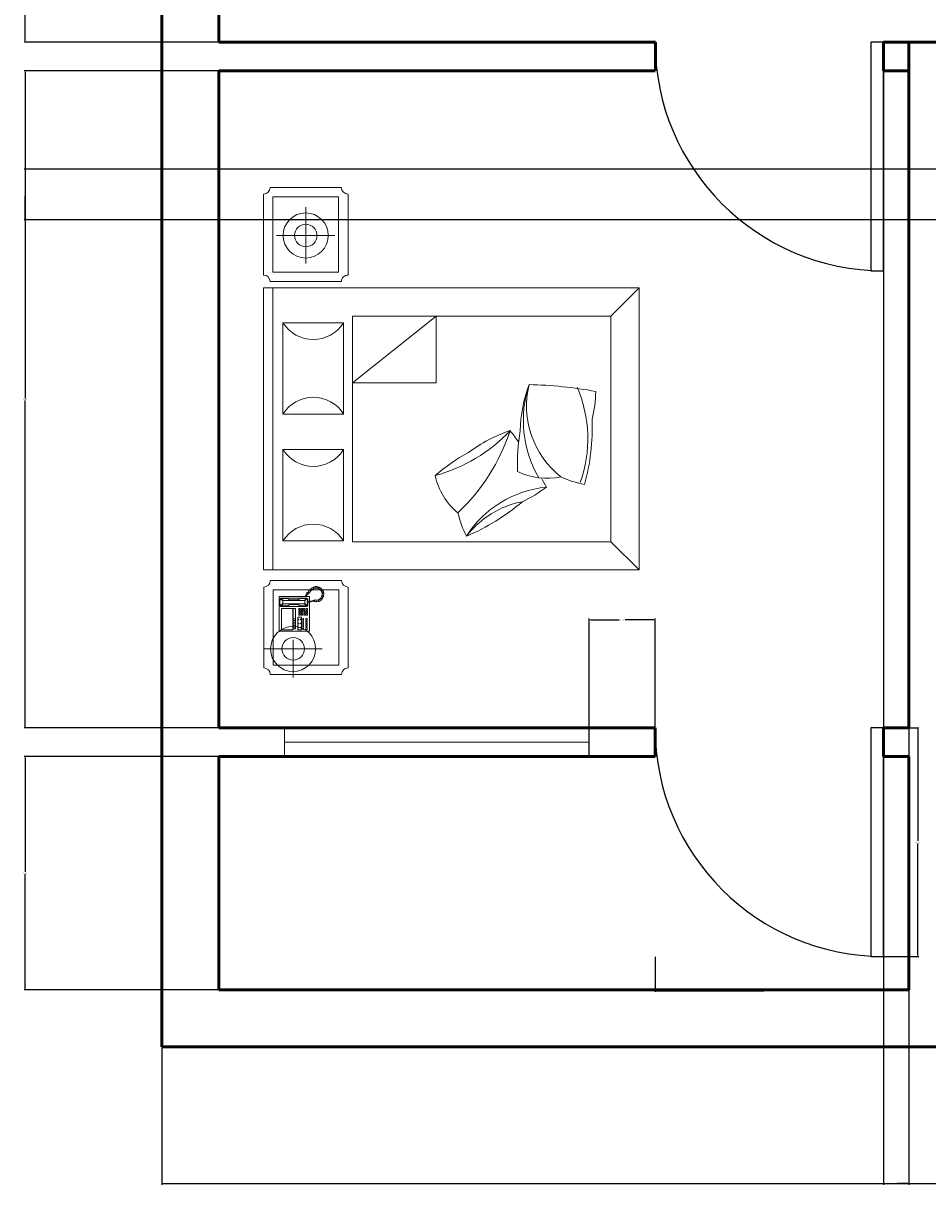
# Model space of a CAD drawing. Units: inches. Extents: x -108 to 1456, y -102 to 617.
# Tile 2 of 8: x 205 to 347, y 154 to 337. Entities that reach past the tile are written whole.
import ezdxf

# ---------------------------------------------------------------- set-up
doc = ezdxf.new("R2010")
doc.units = ezdxf.units.IN
for name, color, linetype, lineweight in [('A-ANNO-DIMS', 2, 'Continuous', 18), ('A-DOOR', 3, 'Continuous', 25), ('A-FURN', 8, 'Continuous', 18), ('A-GLAZ', 4, 'Continuous', 18), ('A-WALL', 7, 'Continuous', 50)]:
    doc.layers.add(name, color=color, linetype=linetype, lineweight=lineweight)
doc.styles.get("Standard").update_dxf_attribs({"font": 'arial.ttf'})
doc.dimstyles.get("Standard").update_dxf_attribs({"dimtxt": 0.18, "dimasz": 0.18, "dimexe": 0.18, "dimexo": 0.0625, "dimgap": 0.09, "dimtad": 0, "dimtih": 1, "dimtoh": 1, "dimdec": 4, "dimzin": 0, "dimdsep": 46, "dimtxsty": 'Standard', "dimcen": 0.09, "dimadec": 0, "dimazin": 0, "dimtfac": 1, "dimtdec": 4, "dimtofl": 0, "dimtmove": 0, "dimatfit": 3, "dimfxl": 1, "dimtolj": 1, "dimtzin": 0, "dimarcsym": 0})

# ---------------------------------------------------------------- blocks, each defined once
blk = doc.blocks.new('A$C50B66110')
for p, q in [((0.0503, 1.9981), (0.4803, 1.9981)), ((0.1513, 1.6871), (0.1513, 1.9967)), ((0.5716, 1.9488), (0.5716, 2)), ((0.5716, 2), (2.0719, 2)), ((2.0719, 1.9488), (2.0719, 2)), ((2.5701, 1.9993), (2.1401, 1.9993)), ((0.0153, 1.9631), (0.0153, 1.5831)), ((0.0653, 1.9481), (0.0653, 1.5981)), ((0.0653, 1.9481), (0.4653, 1.9481)), ((0.4653, 1.9481), (0.4653, 1.5981)), ((0.5153, 1.9631), (0.5153, 1.5831)), ((2.0719, 1.9488), (0.5716, 1.9488)), ((0.5716, 1.9488), (0.5716, 0)), ((2.0719, 0), (2.0719, 1.9488)), ((2.1051, 1.9643), (2.1051, 1.5843)), ((2.1551, 1.9493), (2.1551, 1.5993)), ((2.5551, 1.9493), (2.1551, 1.9493)), ((2.3505, 1.62), (2.3505, 1.9295)), ((2.5551, 1.9493), (2.5551, 1.5993)), ((2.6051, 1.9643), (2.6051, 1.5843)), ((0.7257, 1.5725), (0.7257, 1.8954)), ((0.7257, 1.8954), (1.2113, 1.8954)), ((1.2113, 1.8954), (1.2113, 1.5725)), ((1.4007, 1.5725), (1.4007, 1.8954)), ((1.4007, 1.8954), (1.8863, 1.8954)), ((1.8863, 1.8954), (1.8863, 1.5725)), ((0, 1.8416), (0.2001, 1.8416)), ((2.5018, 1.7744), (2.2017, 1.7744)), ((0.0503, 1.5481), (0.4803, 1.5481)), ((0.0653, 1.5981), (0.4653, 1.5981)), ((1.2113, 1.5725), (0.7257, 1.5725)), ((1.8863, 1.5725), (1.4007, 1.5725)), ((2.5701, 1.5493), (2.1401, 1.5493)), ((2.5551, 1.5993), (2.1551, 1.5993)), ((1.5665, 1.5254), (1.5665, 1.0802)), ((1.5665, 1.5254), (1.9219, 1.0802)), ((1.9219, 1.0802), (1.5665, 1.0802)), ((0.5716, 0), (0.7216, 0.15)), ((2.0719, 0), (1.9219, 0.15)), ((0.5716, 0), (2.0719, 0))]:
    blk.add_line(p, q)
at = {"linetype": 'ByBlock'}
for p, q in [((0.2481, 1.9162), (0.2458, 1.9139)), ((0.2481, 1.9162), (0.4287, 1.9162)), ((0.4287, 1.9162), (0.4309, 1.9139)), ((0.2458, 1.9139), (0.2458, 1.7562)), ((0.2526, 1.9036), (0.2526, 1.8431)), ((0.3669, 1.9036), (0.2526, 1.9036)), ((0.3669, 1.8431), (0.3669, 1.9036)), ((0.3772, 1.9071), (0.3818, 1.9128)), ((0.3772, 1.7688), (0.3772, 1.9071)), ((0.3818, 1.9094), (0.3807, 1.9048)), ((0.3807, 1.9048), (0.3807, 1.8739)), ((0.3807, 1.9048), (0.3909, 1.8945)), ((0.3807, 1.8739), (0.3829, 1.8682)), ((0.3818, 1.9128), (0.4161, 1.9128)), ((0.3864, 1.9116), (0.3818, 1.9094)), ((0.3829, 1.8682), (0.3864, 1.8625)), ((0.3921, 1.8968), (0.3864, 1.9116)), ((0.3864, 1.9116), (0.4138, 1.9116)), ((0.3864, 1.8625), (0.3875, 1.8545)), ((0.3875, 1.8545), (0.3875, 1.8431)), ((0.3909, 1.8945), (0.3921, 1.8968)), ((0.3909, 1.8431), (0.3909, 1.8945)), ((0.4081, 1.8968), (0.3921, 1.8968)), ((0.4081, 1.8968), (0.4138, 1.9116)), ((0.4092, 1.8945), (0.4081, 1.8968)), ((0.4195, 1.9048), (0.4092, 1.8945)), ((0.4092, 1.8431), (0.4092, 1.8945)), ((0.4138, 1.8625), (0.4127, 1.8545)), ((0.4127, 1.8545), (0.4127, 1.8431)), ((0.4138, 1.9116), (0.4184, 1.9094)), ((0.4172, 1.8682), (0.4138, 1.8625)), ((0.4161, 1.9128), (0.4218, 1.9071)), ((0.4195, 1.8739), (0.4172, 1.8682)), ((0.4184, 1.9094), (0.4195, 1.9048)), ((0.4195, 1.9048), (0.4195, 1.8739)), ((0.4218, 1.9071), (0.4218, 1.7699)), ((0.4309, 1.9139), (0.4309, 1.7562)), ((0.2526, 1.8431), (0.3669, 1.8431)), ((0.3201, 1.8168), (0.2526, 1.8168)), ((0.2526, 1.8168), (0.2526, 1.7962)), ((0.2526, 1.7962), (0.3201, 1.7962)), ((0.2572, 1.8408), (0.2572, 1.8294)), ((0.3669, 1.8408), (0.2572, 1.8408)), ((0.2572, 1.8294), (0.3669, 1.8294)), ((0.2675, 1.8145), (0.2641, 1.8145)), ((0.2641, 1.8145), (0.2641, 1.8111)), ((0.2641, 1.8111), (0.2675, 1.8111)), ((0.2641, 1.8019), (0.2641, 1.7985)), ((0.2675, 1.8019), (0.2641, 1.8019)), ((0.2641, 1.7985), (0.2675, 1.7985)), ((0.2664, 1.8408), (0.2664, 1.8294)), ((0.2675, 1.8111), (0.2675, 1.8145)), ((0.2675, 1.7985), (0.2675, 1.8019)), ((0.2755, 1.8408), (0.2755, 1.8294)), ((0.2846, 1.8408), (0.2846, 1.8294)), ((0.2846, 1.8145), (0.2846, 1.8111)), ((0.2881, 1.8145), (0.2846, 1.8145)), ((0.2846, 1.8111), (0.2881, 1.8111)), ((0.2846, 1.8019), (0.2846, 1.7985)), ((0.2881, 1.8019), (0.2846, 1.8019)), ((0.2846, 1.7985), (0.2881, 1.7985)), ((0.2881, 1.8111), (0.2881, 1.8145)), ((0.2881, 1.7985), (0.2881, 1.8019)), ((0.2938, 1.8408), (0.2938, 1.8294)), ((0.3029, 1.8408), (0.3029, 1.8294)), ((0.3052, 1.8145), (0.3052, 1.8111)), ((0.3086, 1.8145), (0.3052, 1.8145)), ((0.3052, 1.8111), (0.3086, 1.8111)), ((0.3052, 1.8019), (0.3052, 1.7985)), ((0.3086, 1.8019), (0.3052, 1.8019)), ((0.3052, 1.7985), (0.3086, 1.7985)), ((0.3086, 1.8111), (0.3086, 1.8145)), ((0.3086, 1.7985), (0.3086, 1.8019)), ((0.3121, 1.8408), (0.3121, 1.8294)), ((0.3201, 1.7962), (0.3201, 1.8168)), ((0.3304, 1.8111), (0.3395, 1.8111)), ((0.3304, 1.8042), (0.3304, 1.8111)), ((0.3395, 1.8042), (0.3304, 1.8042)), ((0.3304, 1.7985), (0.3395, 1.7985)), ((0.3304, 1.7916), (0.3304, 1.7985)), ((0.3395, 1.8111), (0.3395, 1.8042)), ((0.3395, 1.7985), (0.3395, 1.7916)), ((0.3441, 1.8042), (0.3441, 1.8111)), ((0.3441, 1.8111), (0.3532, 1.8111)), ((0.3532, 1.8042), (0.3441, 1.8042)), ((0.3441, 1.7985), (0.3532, 1.7985)), ((0.3441, 1.7916), (0.3441, 1.7985)), ((0.3532, 1.8111), (0.3532, 1.8042)), ((0.3532, 1.7985), (0.3532, 1.7916)), ((0.3578, 1.8111), (0.3669, 1.8111)), ((0.3578, 1.8042), (0.3578, 1.8111)), ((0.3669, 1.8042), (0.3578, 1.8042)), ((0.3578, 1.7985), (0.3669, 1.7985)), ((0.3578, 1.7916), (0.3578, 1.7985)), ((0.3669, 1.8294), (0.3669, 1.8408)), ((0.3669, 1.8111), (0.3669, 1.8042)), ((0.3669, 1.7985), (0.3669, 1.7916)), ((0.3807, 1.8019), (0.3829, 1.8076)), ((0.3807, 1.7711), (0.3807, 1.8019)), ((0.3829, 1.8076), (0.3864, 1.8134)), ((0.3864, 1.8134), (0.3875, 1.8214)), ((0.3875, 1.8214), (0.3875, 1.8431)), ((0.3909, 1.8431), (0.3909, 1.7813)), ((0.4092, 1.8431), (0.4092, 1.7813)), ((0.4127, 1.8214), (0.4127, 1.8431)), ((0.4138, 1.8134), (0.4127, 1.8214)), ((0.4172, 1.8076), (0.4138, 1.8134)), ((0.4195, 1.8019), (0.4172, 1.8076)), ((0.4195, 1.7711), (0.4195, 1.8019)), ((0.2458, 1.7562), (0.2481, 1.7539)), ((0.4, 1.7539), (0.2481, 1.7539)), ((0.2652, 1.7905), (0.2538, 1.7905)), ((0.2538, 1.7905), (0.2538, 1.7859)), ((0.2538, 1.7859), (0.2652, 1.7859)), ((0.2538, 1.7665), (0.2538, 1.7733)), ((0.2538, 1.7733), (0.2652, 1.7733)), ((0.2652, 1.7665), (0.2538, 1.7665)), ((0.2652, 1.7859), (0.2652, 1.7905)), ((0.2652, 1.7733), (0.2652, 1.7665)), ((0.2812, 1.7905), (0.2698, 1.7905)), ((0.2698, 1.7905), (0.2698, 1.7859)), ((0.2698, 1.7859), (0.2812, 1.7859)), ((0.2698, 1.7665), (0.2698, 1.7733)), ((0.2698, 1.7733), (0.2812, 1.7733)), ((0.2812, 1.7665), (0.2698, 1.7665)), ((0.2812, 1.7859), (0.2812, 1.7905)), ((0.2812, 1.7733), (0.2812, 1.7665)), ((0.2972, 1.7905), (0.2858, 1.7905)), ((0.2858, 1.7905), (0.2858, 1.7859)), ((0.2858, 1.7859), (0.2972, 1.7859)), ((0.2858, 1.7665), (0.2858, 1.7733)), ((0.2858, 1.7733), (0.2972, 1.7733)), ((0.2972, 1.7665), (0.2858, 1.7665)), ((0.2972, 1.7859), (0.2972, 1.7905)), ((0.2972, 1.7733), (0.2972, 1.7665)), ((0.3018, 1.7905), (0.3018, 1.7859)), ((0.3132, 1.7905), (0.3018, 1.7905)), ((0.3018, 1.7859), (0.3132, 1.7859)), ((0.3018, 1.7733), (0.3132, 1.7733)), ((0.3018, 1.7665), (0.3018, 1.7733)), ((0.3132, 1.7665), (0.3018, 1.7665)), ((0.3132, 1.7859), (0.3132, 1.7905)), ((0.3132, 1.7733), (0.3132, 1.7665)), ((0.3395, 1.7916), (0.3304, 1.7916)), ((0.3304, 1.7779), (0.3304, 1.7848)), ((0.3304, 1.7848), (0.3395, 1.7848)), ((0.3395, 1.7779), (0.3304, 1.7779)), ((0.3304, 1.7722), (0.3395, 1.7722)), ((0.3304, 1.7653), (0.3304, 1.7722)), ((0.3395, 1.7653), (0.3304, 1.7653)), ((0.3395, 1.7848), (0.3395, 1.7779)), ((0.3395, 1.7722), (0.3395, 1.7653)), ((0.3532, 1.7916), (0.3441, 1.7916)), ((0.3441, 1.7779), (0.3441, 1.7848)), ((0.3441, 1.7848), (0.3532, 1.7848)), ((0.3532, 1.7779), (0.3441, 1.7779)), ((0.3441, 1.7722), (0.3532, 1.7722)), ((0.3441, 1.7653), (0.3441, 1.7722)), ((0.3532, 1.7653), (0.3441, 1.7653)), ((0.3532, 1.7848), (0.3532, 1.7779)), ((0.3532, 1.7722), (0.3532, 1.7653)), ((0.3669, 1.7916), (0.3578, 1.7916)), ((0.3578, 1.7791), (0.3578, 1.7859)), ((0.3578, 1.7859), (0.3669, 1.7859)), ((0.3669, 1.7791), (0.3578, 1.7791)), ((0.3578, 1.7653), (0.3578, 1.7722)), ((0.3578, 1.7722), (0.3669, 1.7722)), ((0.3669, 1.7653), (0.3578, 1.7653)), ((0.3669, 1.7859), (0.3669, 1.7791)), ((0.3669, 1.7722), (0.3669, 1.7653)), ((0.3829, 1.7631), (0.3772, 1.7688)), ((0.3807, 1.7711), (0.3909, 1.7813)), ((0.3818, 1.7665), (0.3807, 1.7711)), ((0.3864, 1.7642), (0.3818, 1.7665)), ((0.399, 1.7631), (0.3829, 1.7631)), ((0.3921, 1.7791), (0.3864, 1.7642)), ((0.3864, 1.7642), (0.399, 1.7642)), ((0.3909, 1.7813), (0.3921, 1.7791)), ((0.4081, 1.7791), (0.3921, 1.7791)), ((0.4024, 1.7676), (0.3989, 1.7676)), ((0.3989, 1.7676), (0.3991, 1.7578)), ((0.3991, 1.7578), (0.4019, 1.7462)), ((0.4019, 1.7462), (0.4047, 1.7353)), ((0.403, 1.7585), (0.4024, 1.7676)), ((0.4026, 1.7642), (0.4138, 1.7642)), ((0.4161, 1.7631), (0.4027, 1.7631)), ((0.4047, 1.7511), (0.403, 1.7585)), ((0.4287, 1.7539), (0.404, 1.7539)), ((0.4047, 1.7353), (0.4044, 1.7293)), ((0.4074, 1.7402), (0.4047, 1.7511)), ((0.4081, 1.7346), (0.4074, 1.7402)), ((0.4079, 1.7286), (0.4081, 1.7346)), ((0.4092, 1.7813), (0.4081, 1.7791)), ((0.4081, 1.7791), (0.4138, 1.7642)), ((0.4195, 1.7711), (0.4092, 1.7813)), ((0.4138, 1.7642), (0.4184, 1.7665)), ((0.4218, 1.7699), (0.4161, 1.7631)), ((0.4184, 1.7665), (0.4195, 1.7711)), ((0.4309, 1.7562), (0.4287, 1.7539)), ((0.4378, 1.7742), (0.4309, 1.7768)), ((0.4309, 1.7722), (0.436, 1.7708)), ((0.436, 1.7708), (0.4406, 1.7672)), ((0.441, 1.771), (0.4378, 1.7742)), ((0.4406, 1.7672), (0.4418, 1.7656)), ((0.4434, 1.7688), (0.441, 1.771)), ((0.4443, 1.7658), (0.4418, 1.7633)), ((0.4418, 1.7656), (0.4443, 1.7658)), ((0.4418, 1.7633), (0.4511, 1.7551)), ((0.4477, 1.7704), (0.4434, 1.7688)), ((0.4497, 1.7684), (0.4477, 1.7704)), ((0.4481, 1.765), (0.4497, 1.7684)), ((0.4509, 1.7672), (0.4481, 1.765)), ((0.4539, 1.764), (0.4509, 1.7672)), ((0.4511, 1.7551), (0.4662, 1.7422)), ((0.4515, 1.7573), (0.4539, 1.764)), ((0.4577, 1.7605), (0.4515, 1.7573)), ((0.463, 1.7555), (0.4577, 1.7605)), ((0.4618, 1.7482), (0.463, 1.7555)), ((0.467, 1.7515), (0.4618, 1.7482)), ((0.4664, 1.7418), (0.4741, 1.72)), ((0.4714, 1.7468), (0.467, 1.7515)), ((0.4696, 1.7418), (0.4714, 1.7468)), ((0.4766, 1.7425), (0.4697, 1.7418)), ((0.472, 1.733), (0.4787, 1.7356)), ((0.4794, 1.7332), (0.472, 1.733)), ((0.4787, 1.7356), (0.4766, 1.7425)), ((0.481, 1.7279), (0.4794, 1.7332)), ((0.4026, 1.7254), (0.4021, 1.7198)), ((0.4021, 1.7198), (0.4088, 1.7187)), ((0.4088, 1.7187), (0.4023, 1.7147)), ((0.4023, 1.7147), (0.4028, 1.7085)), ((0.4051, 1.7279), (0.4026, 1.7254)), ((0.4028, 1.7085), (0.4102, 1.7078)), ((0.4102, 1.7078), (0.4037, 1.7027)), ((0.4037, 1.7027), (0.4067, 1.6974)), ((0.4044, 1.7293), (0.4051, 1.7279)), ((0.4067, 1.6974), (0.4137, 1.6988)), ((0.4121, 1.7256), (0.4079, 1.7286)), ((0.4137, 1.6988), (0.4104, 1.6923)), ((0.4104, 1.6923), (0.4139, 1.6881)), ((0.4111, 1.7203), (0.4121, 1.7256)), ((0.4123, 1.7057), (0.4111, 1.7203)), ((0.4211, 1.6946), (0.4123, 1.7057)), ((0.4139, 1.6881), (0.4192, 1.692)), ((0.4192, 1.692), (0.4183, 1.6858)), ((0.4183, 1.6858), (0.4227, 1.683)), ((0.4333, 1.6881), (0.4211, 1.6946)), ((0.4227, 1.683), (0.4283, 1.6876)), ((0.4283, 1.6876), (0.4276, 1.68)), ((0.4276, 1.68), (0.4324, 1.6786)), ((0.4324, 1.6786), (0.4354, 1.6849)), ((0.4472, 1.6869), (0.4333, 1.6881)), ((0.4354, 1.6849), (0.4382, 1.6786)), ((0.4382, 1.6786), (0.4421, 1.6782)), ((0.4421, 1.6782), (0.4437, 1.6849)), ((0.4437, 1.6849), (0.4463, 1.6775)), ((0.4463, 1.6775), (0.4507, 1.6786)), ((0.4606, 1.6927), (0.4472, 1.6869)), ((0.4507, 1.6786), (0.4509, 1.6849)), ((0.4509, 1.6849), (0.4562, 1.6802)), ((0.4562, 1.6802), (0.4599, 1.6821)), ((0.4592, 1.689), (0.4641, 1.683)), ((0.4599, 1.6821), (0.4592, 1.689)), ((0.4708, 1.7027), (0.4606, 1.6927)), ((0.4641, 1.683), (0.4678, 1.6863)), ((0.465, 1.6925), (0.4715, 1.6897)), ((0.4678, 1.6863), (0.465, 1.6925)), ((0.4741, 1.72), (0.4708, 1.7027)), ((0.4745, 1.6925), (0.4713, 1.6988)), ((0.4713, 1.6988), (0.478, 1.6967)), ((0.4715, 1.6897), (0.4745, 1.6925)), ((0.4743, 1.7075), (0.4815, 1.7073)), ((0.4798, 1.7013), (0.4743, 1.7075)), ((0.4761, 1.7233), (0.481, 1.7279)), ((0.4824, 1.7233), (0.4761, 1.7233)), ((0.4764, 1.7154), (0.4835, 1.7175)), ((0.4824, 1.7119), (0.4764, 1.7154)), ((0.478, 1.6967), (0.4798, 1.7013)), ((0.4815, 1.7073), (0.4824, 1.7119)), ((0.4835, 1.7175), (0.4824, 1.7233)), ((0.7216, 1.5254), (1.9219, 1.5254)), ((0.7216, 1.5254), (0.7216, 0.15)), ((1.9219, 0.15), (1.9219, 1.5254)), ((0.7216, 0.15), (1.9219, 0.15))]:
    blk.add_line(p, q, dxfattribs=at)
for centre, radius in [((0.1513, 1.8416), 0.12), ((0.1513, 1.8416), 0.06), ((2.3505, 1.7744), 0.12), ((2.3505, 1.7744), 0.06)]:
    blk.add_circle(centre, radius)
for centre, radius, start, end in [((0.0153, 1.9981), 0.035, 270, 0), ((0.5153, 1.9981), 0.035, 180, 270), ((2.1051, 1.9993), 0.035, 270, 0), ((2.6051, 1.9993), 0.035, 180, 270), ((0.6244, 1.734), 0.1906, 302.12017, 57.87983), ((1.3126, 1.734), 0.1906, 122.12017, 237.87983), ((1.2994, 1.734), 0.1906, 302.12017, 57.87983), ((1.9876, 1.734), 0.1906, 122.12017, 237.87983), ((0.0153, 1.5481), 0.035, 0, 90), ((0.5153, 1.5481), 0.035, 90, 180), ((2.1051, 1.5493), 0.035, 0, 90), ((2.6051, 1.5493), 0.035, 90, 180), ((1.1502, 0.7366), 0.3575, 102.47819, 140.46254), ((0.328, 0.4368), 0.9879, 28.49711, 41.05657), ((1.9117, 1.3157), 0.8697, 195.33601, 226.41927), ((0.9996, 0.4307), 0.548, 103.20343, 117.03623), ((1.656, 1.7093), 1.0798, 223.63057, 251.4288), ((0.4482, 0.4408), 0.5655, 5.33912, 57.68949), ((1.8226, 1.3753), 1.1652, 203.06416, 220.32086), ((0.4548, 0.5307), 0.4879, 10.69865, 52.68638), ((0.5648, 0.4378), 0.7874, 18.35266, 36.68512), ((-0.0179, 2.4352), 2.1977, 305.29657, 307.24182), ((1.5981, 0.9345), 0.734, 205.25901, 216.93514), ((1.4166, 0.4903), 0.3575, 154.0418, 192.02615), ((1.1403, -0.3401), 0.9879, 80.06073, 92.62018), ((1.2867, -0.154), 0.7874, 69.91627, 88.24873), ((1.3672, 0.0075), 0.6085, 71.81005, 120.13512), ((1.4431, 0.1219), 0.4774, 76.18494, 142.00166), ((-0.6401, 0.6314), 2.1977, 349.48843, 358.80544), ((-0.0179, 2.4352), 2.1977, 297.92482, 299.3793), ((1.5626, 0.1822), 0.548, 154.76704, 168.59984), ((1.2678, 0.9611), 0.6885, 250.29361, 293.6414), ((1.3343, 1.4141), 1.1652, 254.62778, 271.88448), ((1.5399, 0.9642), 0.734, 256.82263, 268.49876)]:
    blk.add_arc(centre, radius, start, end)
blk = doc.blocks.new('DOOR-36-SWING')
for p, q in [((36, 36), (34, 36)), ((34, 36), (34, 0)), ((36, 36), (34, 36)), ((36, 0), (36, 36)), ((34, 0), (36, 0))]:
    blk.add_line(p, q)
blk.add_arc((36, 36), 36, 180, 270)
blk = doc.blocks.new('WIN-48-WALL-4_5')
for p, q in [((0, 0), (0, 4.5)), ((48, 0), (48, 4.5)), ((0, 2.25), (48, 2.25))]:
    blk.add_line(p, q)
blk = doc.blocks.new('*D12')
at = {"layer": 'A-ANNO-DIMS', "color": 0, "lineweight": -2, "transparency": 16777216}
for p, q in [((304.09, 189.96), (304.09, 184.44)), ((340.09, 189.96), (340.09, 184.44)), ((304.27, 184.62), (321.16, 184.62)), ((339.91, 184.62), (323.03, 184.62))]:
    blk.add_line(p, q, dxfattribs=at)
at = {"layer": 'A-ANNO-DIMS', "color": 0, "transparency": 16777216}
for points in [[(304.27, 184.65), (304.27, 184.59), (304.09, 184.62)], [(339.91, 184.65), (339.91, 184.59), (340.09, 184.62)]]:
    blk.add_solid(points, dxfattribs=at)
at = {"layer": 'Defpoints', "color": 0, "transparency": 16777216}
for p in [(304.09, 190.02), (340.09, 190.02), (340.09, 184.62)]:
    blk.add_point(p, dxfattribs=at)
at = {"layer": 'A-ANNO-DIMS', "color": 0, "transparency": 16777216, "insert": (322.09, 184.62), "char_height": 0.18, "attachment_point": 5}
blk.add_mtext('\\A1;DOOR 36 TYP.', dxfattribs=at)
blk = doc.blocks.new('*D13')
at = {"layer": 'A-ANNO-DIMS', "color": 0, "lineweight": -2, "transparency": 16777216}
for p, q in [((340.16, 226.02), (345.67, 226.02)), ((345.49, 225.84), (345.49, 208.21)), ((345.49, 190.2), (345.49, 207.84)), ((340.16, 190.02), (345.67, 190.02))]:
    blk.add_line(p, q, dxfattribs=at)
at = {"layer": 'A-ANNO-DIMS', "color": 0, "transparency": 16777216}
for points in [[(345.46, 225.84), (345.52, 225.84), (345.49, 226.02)], [(345.46, 190.2), (345.52, 190.2), (345.49, 190.02)]]:
    blk.add_solid(points, dxfattribs=at)
at = {"layer": 'Defpoints', "color": 0, "transparency": 16777216}
for p in [(340.09, 226.02), (345.49, 226.02), (340.09, 190.02)]:
    blk.add_point(p, dxfattribs=at)
at = {"layer": 'A-ANNO-DIMS', "color": 0, "transparency": 16777216, "insert": (345.49, 208.02), "char_height": 0.18, "attachment_point": 5}
blk.add_mtext('\\A1;36 TYP.', dxfattribs=at)
blk = doc.blocks.new('*D34')
at = {"layer": 'A-ANNO-DIMS', "color": 0, "lineweight": -2, "transparency": 16777216}
for p, q in [((226.34, 175.71), (226.34, 154.07)), ((538.34, 175.71), (538.34, 154.07)), ((226.52, 154.25), (382.06, 154.25)), ((538.16, 154.25), (382.63, 154.25))]:
    blk.add_line(p, q, dxfattribs=at)
at = {"layer": 'A-ANNO-DIMS', "color": 0, "transparency": 16777216}
for points in [[(226.52, 154.28), (226.52, 154.22), (226.34, 154.25)], [(538.16, 154.28), (538.16, 154.22), (538.34, 154.25)]]:
    blk.add_solid(points, dxfattribs=at)
at = {"layer": 'Defpoints', "color": 0, "transparency": 16777216}
for p in [(226.34, 175.77), (538.34, 175.77), (538.34, 154.25)]:
    blk.add_point(p, dxfattribs=at)
at = {"layer": 'A-ANNO-DIMS', "color": 0, "transparency": 16777216, "insert": (382.34, 154.25), "char_height": 0.18, "attachment_point": 5}
blk.add_mtext('\\A1;312', dxfattribs=at)
blk = doc.blocks.new('*D40')
at = {"layer": 'A-ANNO-DIMS', "color": 0, "lineweight": -2, "transparency": 16777216}
for p, q in [((235.28, 449.52), (204.64, 449.52)), ((204.82, 449.34), (204.82, 391.96)), ((204.82, 334.2), (204.82, 391.59)), ((235.28, 334.02), (204.64, 334.02))]:
    blk.add_line(p, q, dxfattribs=at)
at = {"layer": 'A-ANNO-DIMS', "color": 0, "transparency": 16777216}
for points in [[(204.79, 449.34), (204.85, 449.34), (204.82, 449.52)], [(204.79, 334.2), (204.85, 334.2), (204.82, 334.02)]]:
    blk.add_solid(points, dxfattribs=at)
at = {"layer": 'Defpoints', "color": 0, "transparency": 16777216}
for p in [(235.34, 449.52), (204.82, 334.02), (235.34, 334.02)]:
    blk.add_point(p, dxfattribs=at)
at = {"layer": 'A-ANNO-DIMS', "color": 0, "transparency": 16777216, "insert": (204.82, 391.77), "char_height": 0.18, "attachment_point": 5}
blk.add_mtext('\\A1;115.5', dxfattribs=at)
blk = doc.blocks.new('*D41')
at = {"layer": 'A-ANNO-DIMS', "color": 0, "lineweight": -2, "transparency": 16777216}
for p, q in [((235.28, 329.52), (204.64, 329.52)), ((204.82, 329.34), (204.82, 277.96)), ((204.82, 226.2), (204.82, 277.59)), ((235.28, 226.02), (204.64, 226.02))]:
    blk.add_line(p, q, dxfattribs=at)
at = {"layer": 'A-ANNO-DIMS', "color": 0, "transparency": 16777216}
for points in [[(204.79, 329.34), (204.85, 329.34), (204.82, 329.52)], [(204.79, 226.2), (204.85, 226.2), (204.82, 226.02)]]:
    blk.add_solid(points, dxfattribs=at)
at = {"layer": 'Defpoints', "color": 0, "transparency": 16777216}
for p in [(235.34, 329.52), (204.82, 226.02), (235.34, 226.02)]:
    blk.add_point(p, dxfattribs=at)
at = {"layer": 'A-ANNO-DIMS', "color": 0, "transparency": 16777216, "insert": (204.82, 277.77), "char_height": 0.18, "attachment_point": 5}
blk.add_mtext('\\A1;103.5', dxfattribs=at)
blk = doc.blocks.new('*D42')
at = {"layer": 'A-ANNO-DIMS', "color": 0, "lineweight": -2, "transparency": 16777216}
for p, q in [((235.28, 221.52), (204.64, 221.52)), ((204.82, 221.34), (204.82, 203.33)), ((204.82, 184.95), (204.82, 202.97)), ((235.28, 184.77), (204.64, 184.77))]:
    blk.add_line(p, q, dxfattribs=at)
at = {"layer": 'A-ANNO-DIMS', "color": 0, "transparency": 16777216}
for points in [[(204.79, 221.34), (204.85, 221.34), (204.82, 221.52)], [(204.79, 184.95), (204.85, 184.95), (204.82, 184.77)]]:
    blk.add_solid(points, dxfattribs=at)
at = {"layer": 'Defpoints', "color": 0, "transparency": 16777216}
for p in [(235.34, 221.52), (204.82, 184.77), (235.34, 184.77)]:
    blk.add_point(p, dxfattribs=at)
at = {"layer": 'A-ANNO-DIMS', "color": 0, "transparency": 16777216, "insert": (204.82, 203.15), "char_height": 0.18, "attachment_point": 5}
blk.add_mtext('\\A1;36.75', dxfattribs=at)
blk = doc.blocks.new('*D43')
at = {"layer": 'A-ANNO-DIMS', "color": 0, "lineweight": -2, "transparency": 16777216}
for p, q in [((340.09, 329.46), (340.09, 154.07)), ((344.09, 329.46), (344.09, 154.07)), ((340.27, 154.25), (341.94, 154.25)), ((343.91, 154.25), (342.25, 154.25))]:
    blk.add_line(p, q, dxfattribs=at)
at = {"layer": 'A-ANNO-DIMS', "color": 0, "transparency": 16777216}
for points in [[(340.27, 154.28), (340.27, 154.22), (340.09, 154.25)], [(343.91, 154.28), (343.91, 154.22), (344.09, 154.25)]]:
    blk.add_solid(points, dxfattribs=at)
at = {"layer": 'Defpoints', "color": 0, "transparency": 16777216}
for p in [(340.09, 329.52), (344.09, 329.52), (344.09, 154.25)]:
    blk.add_point(p, dxfattribs=at)
at = {"layer": 'A-ANNO-DIMS', "color": 0, "transparency": 16777216, "insert": (342.09, 154.25), "char_height": 0.18, "attachment_point": 5}
blk.add_mtext('\\A1;4', dxfattribs=at)
blk = doc.blocks.new('*D44')
at = {"layer": 'A-ANNO-DIMS', "color": 0, "lineweight": -2, "transparency": 16777216}
for p, q in [((293.72, 221.59), (293.72, 243.23)), ((293.9, 243.05), (298.45, 243.05)), ((303.91, 243.05), (299.36, 243.05)), ((304.09, 221.59), (304.09, 243.23))]:
    blk.add_line(p, q, dxfattribs=at)
at = {"layer": 'A-ANNO-DIMS', "color": 0, "transparency": 16777216}
for points in [[(293.9, 243.08), (293.9, 243.02), (293.72, 243.05)], [(303.91, 243.08), (303.91, 243.02), (304.09, 243.05)]]:
    blk.add_solid(points, dxfattribs=at)
at = {"layer": 'Defpoints', "color": 0, "transparency": 16777216}
for p in [(304.09, 243.05), (293.72, 221.52), (304.09, 221.52)]:
    blk.add_point(p, dxfattribs=at)
at = {"layer": 'A-ANNO-DIMS', "color": 0, "transparency": 16777216, "insert": (298.91, 243.05), "char_height": 0.18, "attachment_point": 5}
blk.add_mtext('\\A1;10.375', dxfattribs=at)
blk = doc.blocks.new('*D64')
at = {"layer": 'A-ANNO-DIMS', "color": 0, "lineweight": -2, "transparency": 16777216}
for p, q in [((348.53, 314.02), (204.64, 314.02)), ((204.82, 313.84), (204.82, 310.21)), ((204.82, 306.2), (204.82, 309.84)), ((348.53, 306.02), (204.64, 306.02))]:
    blk.add_line(p, q, dxfattribs=at)
at = {"layer": 'A-ANNO-DIMS', "color": 0, "transparency": 16777216}
for points in [[(204.79, 313.84), (204.85, 313.84), (204.82, 314.02)], [(204.79, 306.2), (204.85, 306.2), (204.82, 306.02)]]:
    blk.add_solid(points, dxfattribs=at)
at = {"layer": 'Defpoints', "color": 0, "transparency": 16777216}
for p in [(348.59, 314.02), (204.82, 306.02), (348.59, 306.02)]:
    blk.add_point(p, dxfattribs=at)
at = {"layer": 'A-ANNO-DIMS', "color": 0, "transparency": 16777216, "insert": (204.82, 310.02), "char_height": 0.18, "attachment_point": 5}
blk.add_mtext('\\A1;8', dxfattribs=at)

msp = doc.modelspace()

# ---------------------------------------------------------------- linework, layer by layer
at = {"layer": 'A-WALL'}
for p, q in [((226.3443, 595.7743), (226.3443, 175.7743)), ((235.3443, 334.0243), (235.3443, 449.5243)), ((235.3443, 449.5243), (235.3443, 334.0243)), ((304.0943, 334.0243), (235.3443, 334.0243)), ((304.1647, 334.0243), (304.0943, 334.0243)), ((304.1647, 329.5243), (304.1647, 334.0243)), ((344.0943, 334.0243), (340.0943, 334.0243)), ((340.0943, 329.5243), (340.0943, 334.0243)), ((344.0943, 334.0243), (344.0943, 226.0243)), ((344.0943, 329.5243), (344.0943, 334.0243)), ((344.0943, 334.0243), (348.5943, 334.0243)), ((304.0943, 329.5243), (235.3443, 329.5243)), ((235.3443, 329.5243), (235.3443, 226.0243)), ((344.0943, 329.5243), (340.0943, 329.5243)), ((304.0943, 226.0243), (235.3443, 226.0243)), ((304.0943, 221.5243), (304.0943, 226.0243)), ((344.0943, 226.0243), (340.0943, 226.0243)), ((340.0943, 221.5243), (340.0943, 226.0243)), ((304.0943, 221.5243), (235.3443, 221.5243)), ((235.3443, 221.5243), (304.0943, 221.5243)), ((235.3443, 221.5243), (235.3443, 184.7743)), ((344.0943, 221.5243), (340.0943, 221.5243)), ((344.0943, 221.5243), (344.0943, 184.7743)), ((235.3443, 184.7743), (344.0943, 184.7743)), ((226.3443, 175.7743), (538.3443, 175.7743))]:
    msp.add_line(p, q, dxfattribs=at)

# ---------------------------------------------------------------- block references
at = {"layer": 'A-DOOR'}
for p in [(304.094, 298.024), (304.094, 190.024)]:
    msp.add_blockref('DOOR-36-SWING', p, dxfattribs=at)
at = {"layer": 'A-FURN', "xscale": 29.60830491940187, "yscale": 29.60830491940187, "zscale": 29.60830491940187, "rotation": 89.99999999999991}
msp.add_blockref('A$C50B66110', (301.5751, 233.9822), dxfattribs=at)
at = {"layer": 'A-GLAZ'}
msp.add_blockref('WIN-48-WALL-4_5', (245.719, 221.524), dxfattribs=at)

# ---------------------------------------------------------------- dimensions: what is measured, and where the dimension line sits
at = {"layer": 'A-ANNO-DIMS'}
for base, p1, p2, override, picture, middle in [((204.8193, 334.0243), (235.3443, 449.5243), (235.3443, 334.0243), {"dimdec": 1, "dimlfac": 1, "dimrnd": 0, "dimzin": 0, "dimdsep": 46, "dimlunit": 2}, '*D40', (204.8193, 391.7743)), ((204.8193, 226.0243), (235.3443, 329.5243), (235.3443, 226.0243), {"dimdec": 1, "dimlfac": 1, "dimrnd": 0, "dimzin": 0, "dimdsep": 46, "dimlunit": 2}, '*D41', (204.8193, 277.7743)), ((204.8193, 306.0243), (348.5943, 314.0243), (348.5943, 306.0243), {"dimdec": 0, "dimlfac": 1, "dimrnd": 0, "dimzin": 0, "dimdsep": 46, "dimlunit": 2}, '*D64', (204.8193, 310.0243)), ((204.8193, 184.7743), (235.3443, 221.5243), (235.3443, 184.7743), {"dimdec": 2, "dimlfac": 1, "dimrnd": 0, "dimzin": 0, "dimdsep": 46, "dimlunit": 2}, '*D42', (204.8193, 203.1493))]:
    dim = msp.add_linear_dim(base=base, p1=p1, p2=p2, angle=90, dimstyle='Standard', override=override, dxfattribs=at)
    dim.commit()
    dim.dimension.update_dxf_attribs({"geometry": picture, "text_midpoint": middle})
for base, p1, p2, override, picture, middle in [((344.0943, 154.2493), (340.0943, 329.5243), (344.0943, 329.5243), {"dimdec": 0, "dimlfac": 1, "dimrnd": 0, "dimzin": 0, "dimdsep": 46, "dimlunit": 2}, '*D43', (342.0943, 154.2493)), ((304.0943, 243.0493), (293.7193, 221.5243), (304.0943, 221.5243), {"dimdec": 3, "dimlfac": 1, "dimrnd": 0, "dimzin": 0, "dimdsep": 46, "dimlunit": 2}, '*D44', (298.9068, 243.0493)), ((538.3443, 154.2493), (226.3443, 175.7743), (538.3443, 175.7743), {"dimdec": 0, "dimlfac": 1, "dimrnd": 0, "dimzin": 0, "dimdsep": 46, "dimlunit": 2}, '*D34', (382.3443, 154.2493))]:
    dim = msp.add_linear_dim(base=base, p1=p1, p2=p2, dimstyle='Standard', override=override, dxfattribs=at)
    dim.commit()
    dim.dimension.update_dxf_attribs({"geometry": picture, "text_midpoint": middle})
dim = msp.add_linear_dim(base=(345.4943, 226.0243), p1=(340.0943, 190.0243), p2=(340.0943, 226.0243), angle=90, text='<> TYP.', dimstyle='Standard', override={"dimdec": 0, "dimlfac": 1, "dimrnd": 0, "dimzin": 0, "dimdsep": 46, "dimlunit": 2}, dxfattribs=at)
dim.commit()
dim.dimension.update_dxf_attribs({"geometry": '*D13', "text_midpoint": (345.4943, 208.0243)})
dim = msp.add_linear_dim(base=(340.0943, 184.6243), p1=(304.0943, 190.0243), p2=(340.0943, 190.0243), text='DOOR <> TYP.', dimstyle='Standard', override={"dimdec": 0, "dimlfac": 1, "dimrnd": 0, "dimzin": 0, "dimdsep": 46, "dimlunit": 2}, dxfattribs=at)
dim.commit()
dim.dimension.update_dxf_attribs({"geometry": '*D12', "text_midpoint": (322.0943, 184.6243)})

doc.saveas('drawing.dxf')
